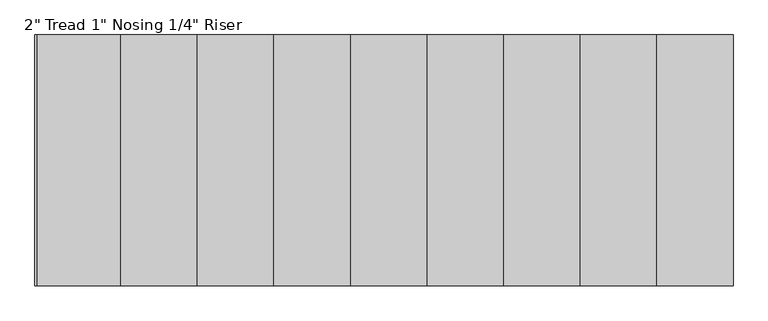
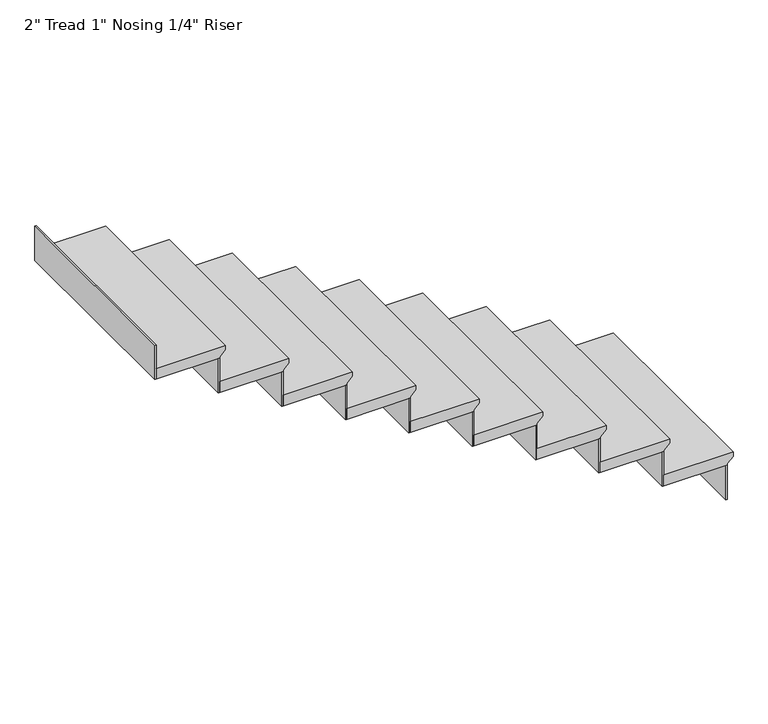
"""IFC4 building model written with IfcOpenShell, lengths in millimetres: stair flight geometry."""

from ifc_helpers import new_model, si_unit, frame, origin, place, context, project, spatial, polyline, outline, extrude, source, transform, mapped, element, save


def stair_flight_1fb61bbc(model_context):
    return source(origin(), model_context, "Body", "SweptSolid", [
        extrude(outline(polyline([(24163.02, 923.4845537), (24163.02, 618.6845537), (24112.22, 618.6845537), (24112.22, 898.0845537), (24118.57, 898.0845537), (24143.97, 923.4845537), (24163.02, 923.4845537)])), frame((0.0, -5753.3544725, 0.0), z_axis=(0.0, 1.0, 0.0), x_axis=(0.0, 0.0, 1.0)), (0.0, 0.0, 1.0), 914.4),
        extrude(outline(polyline([(891.7345537, -4838.9544725), (898.0845537, -4838.9544725), (898.0845537, -5753.3544725), (891.7345537, -5753.3544725), (891.7345537, -4838.9544725)])), frame((0.0, 0.0, 23952.2), z_axis=(0.0, 0.0, 1.0), x_axis=(1.0, 0.0, 0.0)), (0.0, 0.0, 1.0), 160.02),
        extrude(outline(polyline([(612.3345537, -4838.9544725), (618.6845537, -4838.9544725), (618.6845537, -5753.3544725), (612.3345537, -5753.3544725), (612.3345537, -4838.9544725)])), frame((0.0, 0.0, 24112.22), z_axis=(0.0, 0.0, 1.0), x_axis=(1.0, 0.0, 0.0)), (0.0, 0.0, 1.0), 160.02),
        extrude(outline(polyline([(24323.04, 644.0845537), (24323.04, 339.2845537), (24272.24, 339.2845537), (24272.24, 618.6845537), (24278.59, 618.6845537), (24303.99, 644.0845537), (24323.04, 644.0845537)])), frame((0.0, -5753.3544725, 0.0), z_axis=(0.0, 1.0, 0.0), x_axis=(0.0, 0.0, 1.0)), (0.0, 0.0, 1.0), 914.4),
        extrude(outline(polyline([(332.9345537, -4838.9544725), (339.2845537, -4838.9544725), (339.2845537, -5753.3544725), (332.9345537, -5753.3544725), (332.9345537, -4838.9544725)])), frame((0.0, 0.0, 24272.24), z_axis=(0.0, 0.0, 1.0), x_axis=(1.0, 0.0, 0.0)), (0.0, 0.0, 1.0), 160.02),
        extrude(outline(polyline([(24483.06, 364.6845537), (24483.06, 59.8845537), (24432.26, 59.8845537), (24432.26, 339.2845537), (24438.61, 339.2845537), (24464.01, 364.6845537), (24483.06, 364.6845537)])), frame((0.0, -5753.3544725, 0.0), z_axis=(0.0, 1.0, 0.0), x_axis=(0.0, 0.0, 1.0)), (0.0, 0.0, 1.0), 914.4),
        extrude(outline(polyline([(53.5345537, -4838.9544725), (59.8845537, -4838.9544725), (59.8845537, -5753.3544725), (53.5345537, -5753.3544725), (53.5345537, -4838.9544725)])), frame((0.0, 0.0, 24432.26), z_axis=(0.0, 0.0, 1.0), x_axis=(1.0, 0.0, 0.0)), (0.0, 0.0, 1.0), 160.02),
        extrude(outline(polyline([(24643.08, 85.2845537), (24643.08, -219.5154463), (24592.28, -219.5154463), (24592.28, 59.8845537), (24598.63, 59.8845537), (24624.03, 85.2845537), (24643.08, 85.2845537)])), frame((0.0, -5753.3544725, 0.0), z_axis=(0.0, 1.0, 0.0), x_axis=(0.0, 0.0, 1.0)), (0.0, 0.0, 1.0), 914.4),
        extrude(outline(polyline([(-225.8654463, -4838.9544725), (-219.5154463, -4838.9544725), (-219.5154463, -5753.3544725), (-225.8654463, -5753.3544725), (-225.8654463, -4838.9544725)])), frame((0.0, 0.0, 24592.28), z_axis=(0.0, 0.0, 1.0), x_axis=(1.0, 0.0, 0.0)), (0.0, 0.0, 1.0), 160.02),
        extrude(outline(polyline([(24803.1, -194.1154463), (24803.1, -498.9154463), (24752.3, -498.9154463), (24752.3, -219.5154463), (24758.65, -219.5154463), (24784.05, -194.1154463), (24803.1, -194.1154463)])), frame((0.0, -5753.3544725, 0.0), z_axis=(0.0, 1.0, 0.0), x_axis=(0.0, 0.0, 1.0)), (0.0, 0.0, 1.0), 914.4),
        extrude(outline(polyline([(-505.2654463, -4838.9544725), (-498.9154463, -4838.9544725), (-498.9154463, -5753.3544725), (-505.2654463, -5753.3544725), (-505.2654463, -4838.9544725)])), frame((0.0, 0.0, 24752.3), z_axis=(0.0, 0.0, 1.0), x_axis=(1.0, 0.0, 0.0)), (0.0, 0.0, 1.0), 160.02),
        extrude(outline(polyline([(24963.12, -473.5154463), (24963.12, -778.3154463), (24912.32, -778.3154463), (24912.32, -498.9154463), (24918.67, -498.9154463), (24944.07, -473.5154463), (24963.12, -473.5154463)])), frame((0.0, -5753.3544725, 0.0), z_axis=(0.0, 1.0, 0.0), x_axis=(0.0, 0.0, 1.0)), (0.0, 0.0, 1.0), 914.4),
        extrude(outline(polyline([(-784.6654463, -4838.9544725), (-778.3154463, -4838.9544725), (-778.3154463, -5753.3544725), (-784.6654463, -5753.3544725), (-784.6654463, -4838.9544725)])), frame((0.0, 0.0, 24912.32), z_axis=(0.0, 0.0, 1.0), x_axis=(1.0, 0.0, 0.0)), (0.0, 0.0, 1.0), 160.02),
        extrude(outline(polyline([(25123.14, -752.9154463), (25123.14, -1057.7154463), (25072.34, -1057.7154463), (25072.34, -778.3154463), (25078.69, -778.3154463), (25104.09, -752.9154463), (25123.14, -752.9154463)])), frame((0.0, -5753.3544725, 0.0), z_axis=(0.0, 1.0, 0.0), x_axis=(0.0, 0.0, 1.0)), (0.0, 0.0, 1.0), 914.4),
        extrude(outline(polyline([(-1064.0654463, -4838.9544725), (-1057.7154463, -4838.9544725), (-1057.7154463, -5753.3544725), (-1064.0654463, -5753.3544725), (-1064.0654463, -4838.9544725)])), frame((0.0, 0.0, 25072.34), z_axis=(0.0, 0.0, 1.0), x_axis=(1.0, 0.0, 0.0)), (0.0, 0.0, 1.0), 160.02),
        extrude(outline(polyline([(25283.16, -1032.3154463), (25283.16, -1337.1154463), (25232.36, -1337.1154463), (25232.36, -1057.7154463), (25238.71, -1057.7154463), (25264.11, -1032.3154463), (25283.16, -1032.3154463)])), frame((0.0, -5753.3544725, 0.0), z_axis=(0.0, 1.0, 0.0), x_axis=(0.0, 0.0, 1.0)), (0.0, 0.0, 1.0), 914.4),
        extrude(outline(polyline([(-1343.4654463, -4838.9544725), (-1337.1154463, -4838.9544725), (-1337.1154463, -5753.3544725), (-1343.4654463, -5753.3544725), (-1343.4654463, -4838.9544725)])), frame((0.0, 0.0, 25232.36), z_axis=(0.0, 0.0, 1.0), x_axis=(1.0, 0.0, 0.0)), (0.0, 0.0, 1.0), 160.02),
        extrude(outline(polyline([(-1622.8654463, -4838.9544725), (-1616.5154463, -4838.9544725), (-1616.5154463, -5753.3544725), (-1622.8654463, -5753.3544725), (-1622.8654463, -4838.9544725)])), frame((0.0, 0.0, 25392.38), z_axis=(0.0, 0.0, 1.0), x_axis=(1.0, 0.0, 0.0)), (0.0, 0.0, 1.0), 160.02),
        extrude(outline(polyline([(25443.18, -1311.7154463), (25443.18, -1616.5154463), (25392.38, -1616.5154463), (25392.38, -1337.1154463), (25398.73, -1337.1154463), (25424.13, -1311.7154463), (25443.18, -1311.7154463)])), frame((0.0, -5753.3544725, 0.0), z_axis=(0.0, 1.0, 0.0), x_axis=(0.0, 0.0, 1.0)), (0.0, 0.0, 1.0), 914.4),
    ])


if __name__ == "__main__":
    model = new_model("IFC4")
    model_context = context("Model", 3, world=origin())
    ifc_project = project(units=[si_unit("LENGTHUNIT", "METRE", prefix="MILLI")], contexts=[model_context])
    site = spatial("IfcSite", under=ifc_project)
    building = spatial("IfcBuilding", under=site)
    placement = place(None, origin())
    stair_flight_shape = stair_flight_1fb61bbc(model_context)
    element("IfcStairFlight", 1, ObjectType="2\" Tread 1\" Nosing 1/4\" Riser", at=placement, inside=building, context=model_context, shape_type="MappedRepresentation", body=[
        mapped(stair_flight_shape, transform((0.0, 0.0, 0.0), x_axis=(1.0, 0.0, 0.0), y_axis=(0.0, 1.0, 0.0), z_axis=(0.0, 0.0, 1.0))),
    ])
    save(model, "model.ifc")
